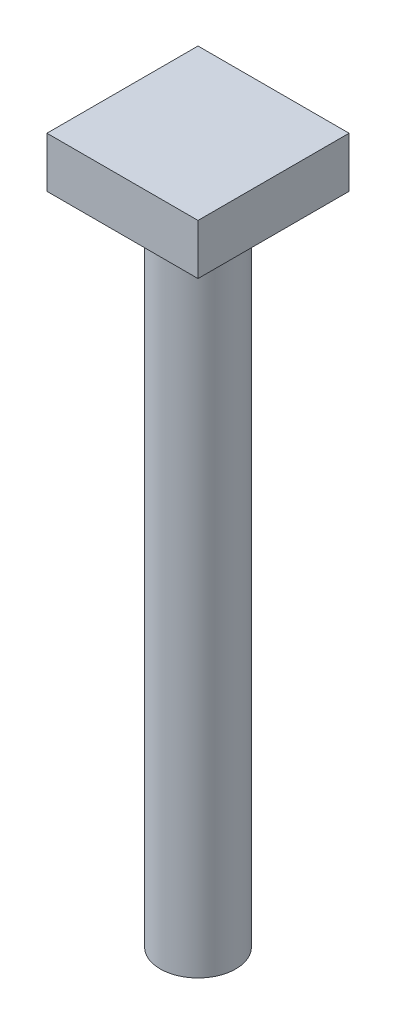
ISO-10303-21;
HEADER;
FILE_DESCRIPTION(('STEP AP214'),'2;1');
FILE_NAME('part.step','',(''),(''),'','','');
FILE_SCHEMA(('AUTOMOTIVE_DESIGN { 1 0 10303 214 1 1 1 1 }'));
ENDSEC;
DATA;
#1=APPLICATION_CONTEXT('core data for automotive mechanical design processes');
#2=APPLICATION_PROTOCOL_DEFINITION('international standard','automotive_design',2000,#1);
#3=PRODUCT_CONTEXT('',#1,'mechanical');
#4=PRODUCT('Part','Part','',(#3));
#5=PRODUCT_RELATED_PRODUCT_CATEGORY('part','',(#4));
#6=PRODUCT_DEFINITION_FORMATION('','',#4);
#7=PRODUCT_DEFINITION_CONTEXT('part definition',#1,'design');
#8=PRODUCT_DEFINITION('design','',#6,#7);
#9=PRODUCT_DEFINITION_SHAPE('','',#8);
#10=(LENGTH_UNIT() NAMED_UNIT(*) SI_UNIT(.MILLI.,.METRE.));
#11=(NAMED_UNIT(*) PLANE_ANGLE_UNIT() SI_UNIT($,.RADIAN.));
#12=(NAMED_UNIT(*) SI_UNIT($,.STERADIAN.) SOLID_ANGLE_UNIT());
#13=UNCERTAINTY_MEASURE_WITH_UNIT(LENGTH_MEASURE(1.E-05),#10,'distance_accuracy_value','');
#14=(GEOMETRIC_REPRESENTATION_CONTEXT(3) GLOBAL_UNCERTAINTY_ASSIGNED_CONTEXT((#13)) GLOBAL_UNIT_ASSIGNED_CONTEXT((#10,
#11,#12)) REPRESENTATION_CONTEXT('',''));
#15=CARTESIAN_POINT('',(0.,0.,0.));
#16=DIRECTION('',(0.,0.,1.));
#17=DIRECTION('',(1.,0.,0.));
#18=AXIS2_PLACEMENT_3D('',#15,#16,#17);
#19=CARTESIAN_POINT('',(12.,8.,-12.));
#20=DIRECTION('',(-1.,0.,0.));
#21=DIRECTION('',(0.,0.,1.));
#22=AXIS2_PLACEMENT_3D('',#19,#20,#21);
#23=PLANE('',#22);
#24=DIRECTION('',(0.,0.,-1.));
#25=VECTOR('',#24,1.);
#26=CARTESIAN_POINT('',(12.,0.,-12.));
#27=LINE('',#26,#25);
#28=CARTESIAN_POINT('',(12.,0.,12.));
#29=VERTEX_POINT('',#28);
#30=CARTESIAN_POINT('',(12.,0.,-12.));
#31=VERTEX_POINT('',#30);
#32=EDGE_CURVE('E102',#29,#31,#27,.T.);
#33=ORIENTED_EDGE('',*,*,#32,.T.);
#34=DIRECTION('',(0.,-1.,0.));
#35=VECTOR('',#34,1.);
#36=CARTESIAN_POINT('',(12.,8.,-12.));
#37=LINE('',#36,#35);
#38=CARTESIAN_POINT('',(12.,8.,-12.));
#39=VERTEX_POINT('',#38);
#40=EDGE_CURVE('E45',#39,#31,#37,.T.);
#41=ORIENTED_EDGE('',*,*,#40,.F.);
#42=DIRECTION('',(0.,0.,-1.));
#43=VECTOR('',#42,1.);
#44=CARTESIAN_POINT('',(12.,8.,-12.));
#45=LINE('',#44,#43);
#46=CARTESIAN_POINT('',(12.,8.,12.));
#47=VERTEX_POINT('',#46);
#48=EDGE_CURVE('E95',#47,#39,#45,.T.);
#49=ORIENTED_EDGE('',*,*,#48,.F.);
#50=DIRECTION('',(0.,-1.,0.));
#51=VECTOR('',#50,1.);
#52=CARTESIAN_POINT('',(12.,8.,12.));
#53=LINE('',#52,#51);
#54=EDGE_CURVE('E103',#47,#29,#53,.T.);
#55=ORIENTED_EDGE('',*,*,#54,.T.);
#56=EDGE_LOOP('',(#33,#41,#49,#55));
#57=FACE_BOUND('',#56,.T.);
#58=ADVANCED_FACE('F39',(#57),#23,.F.);
#59=CARTESIAN_POINT('',(-12.,8.,-12.));
#60=DIRECTION('',(0.,0.,1.));
#61=DIRECTION('',(1.,0.,0.));
#62=AXIS2_PLACEMENT_3D('',#59,#60,#61);
#63=PLANE('',#62);
#64=DIRECTION('',(-1.,0.,0.));
#65=VECTOR('',#64,1.);
#66=CARTESIAN_POINT('',(-12.,0.,-12.));
#67=LINE('',#66,#65);
#68=CARTESIAN_POINT('',(-12.,0.,-12.));
#69=VERTEX_POINT('',#68);
#70=EDGE_CURVE('E97',#31,#69,#67,.T.);
#71=ORIENTED_EDGE('',*,*,#70,.T.);
#72=DIRECTION('',(0.,-1.,0.));
#73=VECTOR('',#72,1.);
#74=CARTESIAN_POINT('',(-12.,8.,-12.));
#75=LINE('',#74,#73);
#76=CARTESIAN_POINT('',(-12.,8.,-12.));
#77=VERTEX_POINT('',#76);
#78=EDGE_CURVE('E92',#77,#69,#75,.T.);
#79=ORIENTED_EDGE('',*,*,#78,.F.);
#80=DIRECTION('',(-1.,0.,0.));
#81=VECTOR('',#80,1.);
#82=CARTESIAN_POINT('',(-12.,8.,-12.));
#83=LINE('',#82,#81);
#84=EDGE_CURVE('E90',#39,#77,#83,.T.);
#85=ORIENTED_EDGE('',*,*,#84,.F.);
#86=ORIENTED_EDGE('',*,*,#40,.T.);
#87=EDGE_LOOP('',(#71,#79,#85,#86));
#88=FACE_BOUND('',#87,.T.);
#89=ADVANCED_FACE('F98',(#88),#63,.F.);
#90=CARTESIAN_POINT('',(-12.,8.,-12.));
#91=DIRECTION('',(1.,0.,0.));
#92=DIRECTION('',(0.,0.,-1.));
#93=AXIS2_PLACEMENT_3D('',#90,#91,#92);
#94=PLANE('',#93);
#95=DIRECTION('',(0.,0.,1.));
#96=VECTOR('',#95,1.);
#97=CARTESIAN_POINT('',(-12.,0.,-12.));
#98=LINE('',#97,#96);
#99=CARTESIAN_POINT('',(-12.,0.,12.));
#100=VERTEX_POINT('',#99);
#101=EDGE_CURVE('E71',#69,#100,#98,.T.);
#102=ORIENTED_EDGE('',*,*,#101,.T.);
#103=DIRECTION('',(0.,-1.,0.));
#104=VECTOR('',#103,1.);
#105=CARTESIAN_POINT('',(-12.,8.,12.));
#106=LINE('',#105,#104);
#107=CARTESIAN_POINT('',(-12.,8.,12.));
#108=VERTEX_POINT('',#107);
#109=EDGE_CURVE('E96',#108,#100,#106,.T.);
#110=ORIENTED_EDGE('',*,*,#109,.F.);
#111=DIRECTION('',(0.,0.,1.));
#112=VECTOR('',#111,1.);
#113=CARTESIAN_POINT('',(-12.,8.,-12.));
#114=LINE('',#113,#112);
#115=EDGE_CURVE('E89',#77,#108,#114,.T.);
#116=ORIENTED_EDGE('',*,*,#115,.F.);
#117=ORIENTED_EDGE('',*,*,#78,.T.);
#118=EDGE_LOOP('',(#102,#110,#116,#117));
#119=FACE_BOUND('',#118,.T.);
#120=ADVANCED_FACE('F100',(#119),#94,.F.);
#121=CARTESIAN_POINT('',(-12.,8.,12.));
#122=DIRECTION('',(0.,0.,-1.));
#123=DIRECTION('',(-1.,0.,0.));
#124=AXIS2_PLACEMENT_3D('',#121,#122,#123);
#125=PLANE('',#124);
#126=DIRECTION('',(1.,0.,0.));
#127=VECTOR('',#126,1.);
#128=CARTESIAN_POINT('',(-12.,0.,12.));
#129=LINE('',#128,#127);
#130=EDGE_CURVE('E79',#100,#29,#129,.T.);
#131=ORIENTED_EDGE('',*,*,#130,.T.);
#132=ORIENTED_EDGE('',*,*,#54,.F.);
#133=DIRECTION('',(1.,0.,0.));
#134=VECTOR('',#133,1.);
#135=CARTESIAN_POINT('',(-12.,8.,12.));
#136=LINE('',#135,#134);
#137=EDGE_CURVE('E57',#108,#47,#136,.T.);
#138=ORIENTED_EDGE('',*,*,#137,.F.);
#139=ORIENTED_EDGE('',*,*,#109,.T.);
#140=EDGE_LOOP('',(#131,#132,#138,#139));
#141=FACE_BOUND('',#140,.T.);
#142=ADVANCED_FACE('F113',(#141),#125,.F.);
#143=CARTESIAN_POINT('',(0.,8.,0.));
#144=DIRECTION('',(0.,1.,0.));
#145=DIRECTION('',(0.,0.,1.));
#146=AXIS2_PLACEMENT_3D('',#143,#144,#145);
#147=PLANE('',#146);
#148=ORIENTED_EDGE('',*,*,#48,.T.);
#149=ORIENTED_EDGE('',*,*,#84,.T.);
#150=ORIENTED_EDGE('',*,*,#115,.T.);
#151=ORIENTED_EDGE('',*,*,#137,.T.);
#152=EDGE_LOOP('',(#148,#149,#150,#151));
#153=FACE_BOUND('',#152,.T.);
#154=ADVANCED_FACE('F88',(#153),#147,.T.);
#155=CARTESIAN_POINT('',(0.,0.,0.));
#156=DIRECTION('',(0.,1.,0.));
#157=DIRECTION('',(0.,0.,1.));
#158=AXIS2_PLACEMENT_3D('',#155,#156,#157);
#159=PLANE('',#158);
#160=CARTESIAN_POINT('',(0.,0.,0.));
#161=DIRECTION('',(0.,-1.,0.));
#162=DIRECTION('',(0.,0.,-1.));
#163=AXIS2_PLACEMENT_3D('',#160,#161,#162);
#164=CIRCLE('',#163,6.);
#165=CARTESIAN_POINT('',(0.,0.,6.));
#166=VERTEX_POINT('',#165);
#167=EDGE_CURVE('E11',#166,#166,#164,.T.);
#168=ORIENTED_EDGE('',*,*,#167,.F.);
#169=EDGE_LOOP('',(#168));
#170=FACE_BOUND('',#169,.T.);
#171=ORIENTED_EDGE('',*,*,#32,.F.);
#172=ORIENTED_EDGE('',*,*,#130,.F.);
#173=ORIENTED_EDGE('',*,*,#101,.F.);
#174=ORIENTED_EDGE('',*,*,#70,.F.);
#175=EDGE_LOOP('',(#171,#172,#173,#174));
#176=FACE_BOUND('',#175,.T.);
#177=ADVANCED_FACE('F116',(#170,#176),#159,.F.);
#178=CARTESIAN_POINT('',(0.,-104.,0.));
#179=DIRECTION('',(0.,1.,0.));
#180=DIRECTION('',(0.,0.,1.));
#181=AXIS2_PLACEMENT_3D('',#178,#179,#180);
#182=CYLINDRICAL_SURFACE('',#181,6.);
#183=CARTESIAN_POINT('',(0.,-104.,0.));
#184=DIRECTION('',(0.,-1.,0.));
#185=DIRECTION('',(0.,0.,-1.));
#186=AXIS2_PLACEMENT_3D('',#183,#184,#185);
#187=CIRCLE('',#186,6.);
#188=CARTESIAN_POINT('',(0.,-104.,6.));
#189=VERTEX_POINT('',#188);
#190=EDGE_CURVE('E108',#189,#189,#187,.T.);
#191=CARTESIAN_POINT('',(0.,-104.,6.));
#192=CARTESIAN_POINT('',(0.,-102.916666666667,6.));
#193=CARTESIAN_POINT('',(0.,-101.833333333333,6.));
#194=CARTESIAN_POINT('',(0.,-99.6666666666667,6.));
#195=CARTESIAN_POINT('',(0.,-98.5833333333333,6.));
#196=CARTESIAN_POINT('',(0.,-96.4166666666667,6.));
#197=CARTESIAN_POINT('',(0.,-95.3333333333333,6.));
#198=CARTESIAN_POINT('',(0.,-93.1666666666666,6.));
#199=CARTESIAN_POINT('',(0.,-92.0833333333333,6.));
#200=CARTESIAN_POINT('',(0.,-89.9166666666667,6.));
#201=CARTESIAN_POINT('',(0.,-88.8333333333333,6.));
#202=CARTESIAN_POINT('',(0.,-86.6666666666667,6.));
#203=CARTESIAN_POINT('',(0.,-85.5833333333333,6.));
#204=CARTESIAN_POINT('',(0.,-83.4166666666667,6.));
#205=CARTESIAN_POINT('',(0.,-82.3333333333333,6.));
#206=CARTESIAN_POINT('',(0.,-80.1666666666666,6.));
#207=CARTESIAN_POINT('',(0.,-79.0833333333333,6.));
#208=CARTESIAN_POINT('',(0.,-76.9166666666666,6.));
#209=CARTESIAN_POINT('',(0.,-75.8333333333333,6.));
#210=CARTESIAN_POINT('',(0.,-73.6666666666667,6.));
#211=CARTESIAN_POINT('',(0.,-72.5833333333333,6.));
#212=CARTESIAN_POINT('',(0.,-70.4166666666667,6.));
#213=CARTESIAN_POINT('',(0.,-69.3333333333333,6.));
#214=CARTESIAN_POINT('',(0.,-67.1666666666667,6.));
#215=CARTESIAN_POINT('',(0.,-66.0833333333333,6.));
#216=CARTESIAN_POINT('',(0.,-63.9166666666667,6.));
#217=CARTESIAN_POINT('',(0.,-62.8333333333333,6.));
#218=CARTESIAN_POINT('',(0.,-60.6666666666667,6.));
#219=CARTESIAN_POINT('',(0.,-59.5833333333333,6.));
#220=CARTESIAN_POINT('',(0.,-57.4166666666667,6.));
#221=CARTESIAN_POINT('',(0.,-56.3333333333333,6.));
#222=CARTESIAN_POINT('',(0.,-54.1666666666667,6.));
#223=CARTESIAN_POINT('',(0.,-53.0833333333333,6.));
#224=CARTESIAN_POINT('',(0.,-50.9166666666667,6.));
#225=CARTESIAN_POINT('',(0.,-49.8333333333333,6.));
#226=CARTESIAN_POINT('',(0.,-47.6666666666667,6.));
#227=CARTESIAN_POINT('',(0.,-46.5833333333333,6.));
#228=CARTESIAN_POINT('',(0.,-44.4166666666667,6.));
#229=CARTESIAN_POINT('',(0.,-43.3333333333333,6.));
#230=CARTESIAN_POINT('',(0.,-41.1666666666667,6.));
#231=CARTESIAN_POINT('',(0.,-40.0833333333333,6.));
#232=CARTESIAN_POINT('',(0.,-37.9166666666667,6.));
#233=CARTESIAN_POINT('',(0.,-36.8333333333333,6.));
#234=CARTESIAN_POINT('',(0.,-34.6666666666667,6.));
#235=CARTESIAN_POINT('',(0.,-33.5833333333333,6.));
#236=CARTESIAN_POINT('',(0.,-31.4166666666667,6.));
#237=CARTESIAN_POINT('',(0.,-30.3333333333333,6.));
#238=CARTESIAN_POINT('',(0.,-28.1666666666667,6.));
#239=CARTESIAN_POINT('',(0.,-27.0833333333333,6.));
#240=CARTESIAN_POINT('',(0.,-24.9166666666667,6.));
#241=CARTESIAN_POINT('',(0.,-23.8333333333333,6.));
#242=CARTESIAN_POINT('',(0.,-21.6666666666667,6.));
#243=CARTESIAN_POINT('',(0.,-20.5833333333333,6.));
#244=CARTESIAN_POINT('',(0.,-18.4166666666667,6.));
#245=CARTESIAN_POINT('',(0.,-17.3333333333333,6.));
#246=CARTESIAN_POINT('',(0.,-15.1666666666667,6.));
#247=CARTESIAN_POINT('',(0.,-14.0833333333333,6.));
#248=CARTESIAN_POINT('',(0.,-11.9166666666667,6.));
#249=CARTESIAN_POINT('',(0.,-10.8333333333333,6.));
#250=CARTESIAN_POINT('',(0.,-8.66666666666666,6.));
#251=CARTESIAN_POINT('',(0.,-7.58333333333333,6.));
#252=CARTESIAN_POINT('',(0.,-5.41666666666667,6.));
#253=CARTESIAN_POINT('',(0.,-4.33333333333334,6.));
#254=CARTESIAN_POINT('',(0.,-2.16666666666667,6.));
#255=CARTESIAN_POINT('',(0.,-1.08333333333333,6.));
#256=CARTESIAN_POINT('',(0.,0.,6.));
#257=B_SPLINE_CURVE_WITH_KNOTS('',3,(#191,#192,#193,#194,#195,#196,#197,#198,#199,#200,#201,
#202,#203,#204,#205,#206,#207,#208,#209,#210,#211,#212,#213,#214,#215,#216,#217,#218,#219,#220,
#221,#222,#223,#224,#225,#226,#227,#228,#229,#230,#231,#232,#233,#234,#235,#236,#237,#238,#239,
#240,#241,#242,#243,#244,#245,#246,#247,#248,#249,#250,#251,#252,#253,#254,#255,#256),
.UNSPECIFIED.,.F.,.F.,(4,2,2,2,2,2,2,2,2,2,2,2,2,2,2,2,2,2,2,2,2,2,2,2,2,2,2,2,2,2,2,2,4),(0.,
3.25,6.50000000000001,9.75000000000001,13.,16.25,19.5,22.75,26.,29.25,32.5,35.75,39.,42.25,45.5,
48.75,52.,55.25,58.5,61.75,65.,68.25,71.5,74.75,78.,81.25,84.5,87.75,91.,94.25,97.5,100.75,
104.),.UNSPECIFIED.);
#258=EDGE_CURVE('BSEAM121',#189,#166,#257,.T.);
#259=ORIENTED_EDGE('',*,*,#190,.F.);
#260=ORIENTED_EDGE('',*,*,#167,.T.);
#261=ORIENTED_EDGE('',*,*,#258,.T.);
#262=ORIENTED_EDGE('',*,*,#258,.F.);
#263=EDGE_LOOP('',(#259,#261,#260,#262));
#264=FACE_BOUND('',#263,.T.);
#265=ADVANCED_FACE('F121',(#264),#182,.T.);
#266=CARTESIAN_POINT('',(0.,-104.,0.));
#267=DIRECTION('',(0.,-1.,0.));
#268=DIRECTION('',(0.,0.,-1.));
#269=AXIS2_PLACEMENT_3D('',#266,#267,#268);
#270=PLANE('',#269);
#271=ORIENTED_EDGE('',*,*,#190,.T.);
#272=EDGE_LOOP('',(#271));
#273=FACE_BOUND('',#272,.T.);
#274=ADVANCED_FACE('F125',(#273),#270,.T.);
#275=CLOSED_SHELL('',(#58,#89,#120,#142,#154,#177,#265,#274));
#276=MANIFOLD_SOLID_BREP('B2',#275);
#277=ADVANCED_BREP_SHAPE_REPRESENTATION('',(#18,#276),#14);
#278=SHAPE_DEFINITION_REPRESENTATION(#9,#277);
ENDSEC;
END-ISO-10303-21;
